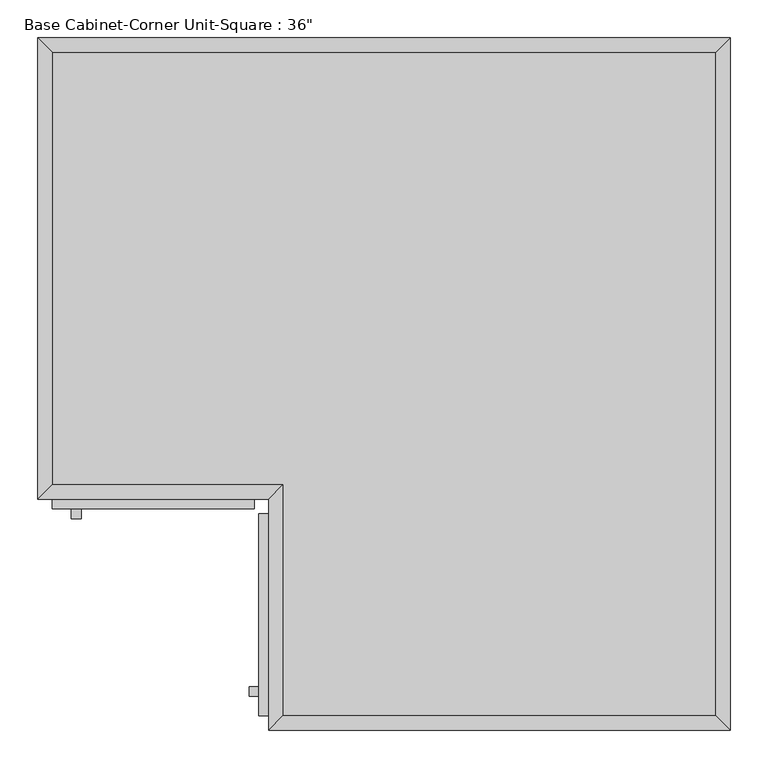
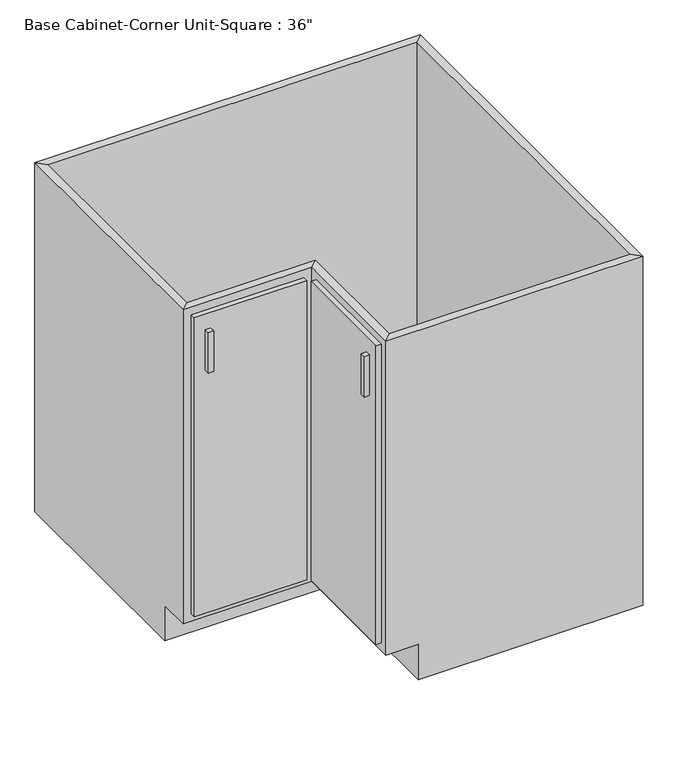
"""IFC4 building model written with IfcOpenShell, lengths in millimetres: furniture geometry."""

from ifc_helpers import new_model, si_unit, frame, origin, place, context, project, spatial, polyline, outline, extrude, faceted_brep, source, transform, mapped, element, save


def furniture_97fe820d(model_context):
    return source(origin(), model_context, "Body", "SolidModel", [
        extrude(outline(polyline([(507.6877049, -19.05), (507.6877049, -895.35), (-63.8122951, -895.35), (-63.8122951, -590.55), (-368.6122951, -590.55), (-368.6122951, -19.05), (507.6877049, -19.05)])), frame((0.0, 0.0, 88.9), z_axis=(0.0, 0.0, 1.0), x_axis=(1.0, 0.0, 0.0)), (0.0, 0.0, 1.0), 19.05),
        extrude(outline(polyline([(-101.9122951, -622.3), (-368.6122951, -622.3), (-368.6122951, -609.6), (-101.9122951, -609.6), (-101.9122951, -622.3)])), frame((0.0, 0.0, 107.95), z_axis=(0.0, 0.0, 1.0), x_axis=(1.0, 0.0, 0.0)), (0.0, 0.0, 1.0), 749.3),
        extrude(outline(polyline([(-330.5122951, -635.0), (-343.2122951, -635.0), (-343.2122951, -622.3), (-330.5122951, -622.3), (-330.5122951, -635.0)])), frame((0.0, 0.0, 717.55), z_axis=(0.0, 0.0, 1.0), x_axis=(1.0, 0.0, 0.0)), (0.0, 0.0, 1.0), 101.6),
        extrude(outline(polyline([(-82.8622951, -628.65), (-82.8622951, -895.35), (-95.5622951, -895.35), (-95.5622951, -628.65), (-82.8622951, -628.65)])), frame((0.0, 0.0, 107.95), z_axis=(0.0, 0.0, 1.0), x_axis=(1.0, 0.0, 0.0)), (0.0, 0.0, 1.0), 749.3),
        extrude(outline(polyline([(-95.5622951, -857.25), (-95.5622951, -869.95), (-108.2622951, -869.95), (-108.2622951, -857.25), (-95.5622951, -857.25)])), frame((0.0, 0.0, 717.55), z_axis=(0.0, 0.0, 1.0), x_axis=(1.0, 0.0, 0.0)), (0.0, 0.0, 1.0), 101.6),
        faceted_brep([(-368.6122951, -533.4, 88.9), (-6.6622951, -533.4, 88.9), (-6.6622951, -895.35, 88.9), (507.6877049, -895.35, 88.9), (507.6877049, -19.05, 88.9), (-368.6122951, -19.05, 88.9), (526.7377049, 0.0, 0.0), (526.7377049, -914.4, 0.0), (-6.6622951, -914.4, 0.0), (-6.6622951, -533.4, 0.0), (-387.6622951, -533.4, 0.0), (-387.6622951, 0.0, 0.0), (-387.6622951, 0.0, 876.3), (526.7377049, 0.0, 876.3), (-387.6622951, -533.4, 88.9), (-387.6622951, -609.6, 88.9), (-387.6622951, -609.6, 876.3), (-6.6622951, -914.4, 88.9), (526.7377049, -914.4, 876.3), (-82.8622951, -914.4, 876.3), (-82.8622951, -914.4, 88.9), (507.6877049, -895.35, 876.3), (-63.8122951, -895.35, 88.9), (-63.8122951, -895.35, 876.3), (-63.8122951, -590.55, 88.9), (-63.8122951, -590.55, 876.3), (-82.8622951, -609.6, 876.3), (-82.8622951, -609.6, 88.9), (-368.6122951, -590.55, 88.9), (-368.6122951, -590.55, 876.3), (-368.6122951, -19.05, 876.3), (507.6877049, -19.05, 876.3)], [[[0, 1, 2, 3, 4, 5]], [[6, 7, 8, 9, 10, 11]], [[6, 11, 12, 13]], [[12, 11, 10, 14, 15, 16]], [[10, 9, 1, 0, 14]], [[9, 8, 17, 2, 1]], [[8, 7, 18, 19, 20, 17]], [[18, 7, 6, 13]], [[21, 3, 2, 22, 23]], [[21, 23, 19, 18]], [[20, 22, 2, 17]], [[23, 22, 24, 25]], [[19, 23, 25, 26]], [[20, 19, 26, 27]], [[22, 20, 27, 24]], [[25, 24, 28, 29]], [[26, 25, 29, 16]], [[27, 26, 16, 15]], [[24, 27, 15, 28]], [[29, 28, 0, 5, 30]], [[16, 29, 30, 12]], [[28, 15, 14, 0]], [[30, 5, 4, 31]], [[12, 30, 31, 13]], [[3, 21, 31, 4]], [[21, 18, 13, 31]]]),
    ])


if __name__ == "__main__":
    model = new_model("IFC4")
    model_context = context("Model", 3, world=origin())
    ifc_project = project(units=[si_unit("LENGTHUNIT", "METRE", prefix="MILLI")], contexts=[model_context])
    site = spatial("IfcSite", under=ifc_project)
    building = spatial("IfcBuilding", under=site)
    placement = place(None, origin())
    furniture_shape = furniture_97fe820d(model_context)
    element("IfcFurniture", 1, ObjectType="Base Cabinet-Corner Unit-Square : 36\"", at=placement, inside=building, context=model_context, shape_type="MappedRepresentation", body=[
        mapped(furniture_shape, transform((0.0, 0.0, 0.0), x_axis=(1.0, 0.0, 0.0), y_axis=(0.0, 1.0, 0.0), z_axis=(0.0, 0.0, 1.0))),
    ])
    save(model, "model.ifc")

# Revit data of these elements
# Type "Base Cabinet-Corner Unit-Square : 36\""
#   Assembly Code = "C1030410"
#   Depth = 2' - 0"
#   Height = 2' - 10 1/2"
#   Toe Depth = 0' - 3"
#   Toe Height = 0' - 3 1/2"
#   Width = 3' - 0"
#   Cabinet Material = Cabinets
#   Door/Drawer Material = Cabinets
#   Handle Material = Cabinets - Handles
#   Default Elevation = 0
# Element 1 (IfcFurniture, "Base Cabinet-Corner Unit-Square : 36\"")
#   Materials on its faces: "Cabinets", "Cabinets - Handles"
# Materials
#   "Cabinets": colour RGB 249 249 249, transparency 0
#   "Cabinets - Handles": colour RGB 57 57 57, transparency 0
